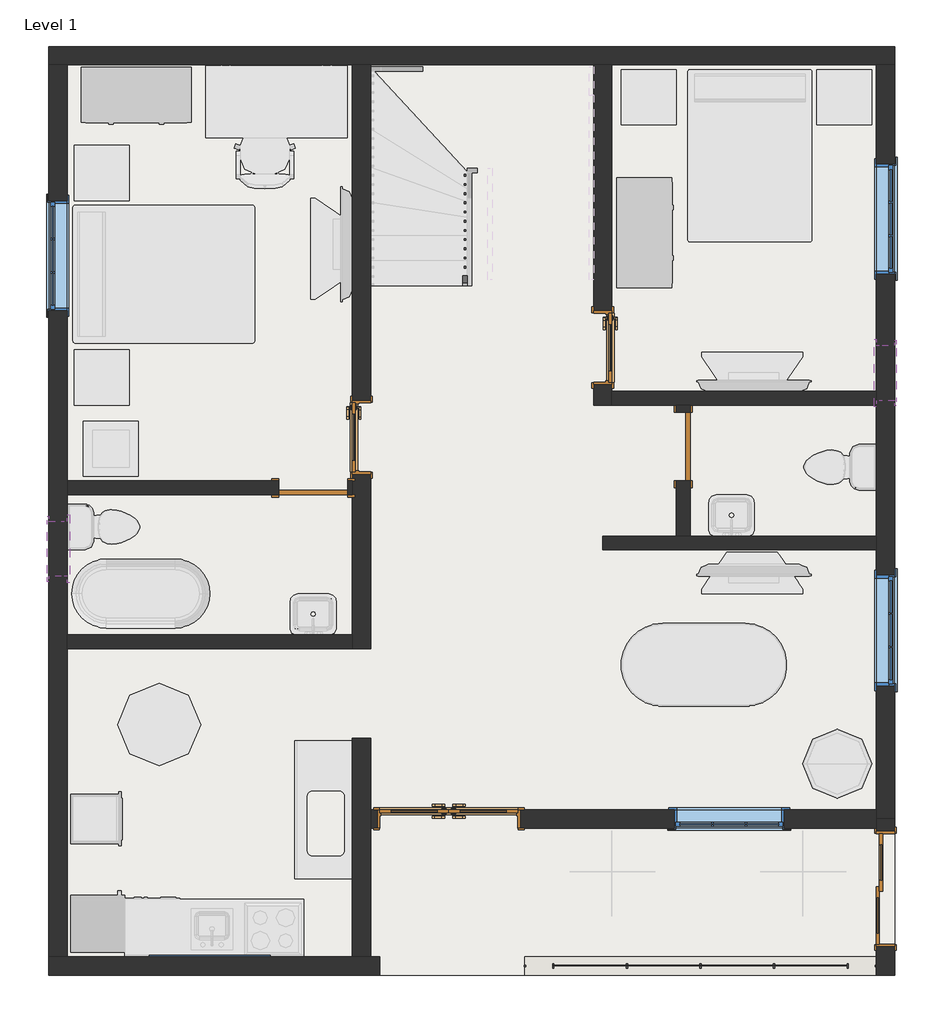
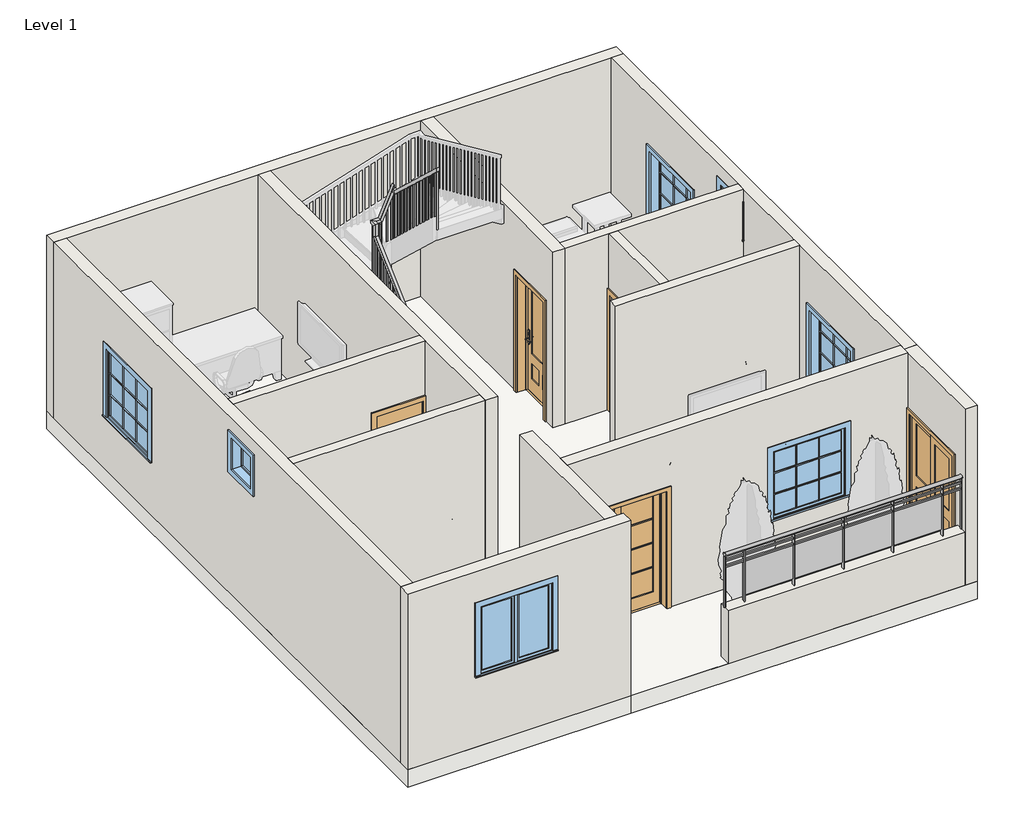
# One storey, part 1 of 2: 15 walls, 7 windows, 6 doors, 2 railings, 1 slab.
"""IFC4 building model written with IfcOpenShell, lengths in millimetres."""

from ifc_helpers import new_model, si_unit, point, frame, origin, origin_with_axes, place, context, project, spatial, polyline, ellipse_curve, trimmed, outline, extrude, faceted_brep, transform, mapped, element, save
from ifc_brep_helpers import plane_surface, extruded_surface, advanced_brep
from components import door_ad59dcae, door_41326d50, door_b03bd389, door_f9cb40a9, door_255cab33, window_3ea3e93d, window_0862ab64, window_e41d21a6

model = new_model("IFC4")

# Units and contexts
model_context = context("Model", 3, world=origin())
ifc_project = project(units=[si_unit("LENGTHUNIT", "METRE", prefix="MILLI")], contexts=[model_context])

# Site, building, storey
site = spatial("IfcSite", under=ifc_project)
building = spatial("IfcBuilding", under=site)
storey = spatial("IfcBuildingStorey", under=building, Name="Level 1", Elevation=0.0)

# Doors
placement = place(None, origin())
door_shape = door_ad59dcae(model_context)
element("IfcDoor", 1, ObjectType="30\" x 80\"", at=placement, inside=storey, context=model_context, shape_type="MappedRepresentation", body=[
    mapped(door_shape, transform((-8446.8361447, 7117.685558, 0.0), x_axis=(0.0, 1.0, 0.0), y_axis=(-1.0, 0.0, 0.0), z_axis=(0.0, 0.0, 1.0))),
])
door_2_shape = door_41326d50(model_context)
element("IfcDoor", 2, ObjectType="30\" x 80\"", at=placement, inside=storey, context=model_context, shape_type="MappedRepresentation", body=[
    mapped(door_2_shape, transform((-5773.4861447, 8108.285558, 0.0), x_axis=(0.0, 1.0, 0.0), y_axis=(-1.0, 0.0, 0.0), z_axis=(0.0, 0.0, 1.0))),
])
door_3_shape = door_b03bd389(model_context)
element("IfcDoor", 3, ObjectType="Door-Exterior-Double-Full Glass-Wood_Clad : 60\" x 80\"", at=placement, inside=storey, context=model_context, shape_type="MappedRepresentation", body=[
    mapped(door_3_shape, transform((-7478.4611447, 2904.460558, 0.0), x_axis=(1.0, 0.0, 0.0), y_axis=(0.0, 1.0, 0.0), z_axis=(0.0, 0.0, 1.0))),
])
door_4_shape = door_f9cb40a9(model_context)
element("IfcDoor", 4, ObjectType="Door-Interior-Double-Sliding-2_Panel-Wood : 48\" x 80\"", at=placement, inside=storey, context=model_context, shape_type="MappedRepresentation", body=[
    mapped(door_4_shape, transform((-2655.6361447, 2126.585558, 0.0), x_axis=(0.0, 1.0, 0.0), y_axis=(-1.0, 0.0, 0.0), z_axis=(0.0, 0.0, 1.0))),
])
door_5_shape = door_255cab33(model_context)
element("IfcDoor", 5, ObjectType="Single-Flush : 30\" x 80\"", at=placement, inside=storey, context=model_context, shape_type="MappedRepresentation", body=[
    mapped(door_5_shape, transform((-8977.0611447, 6558.885558, 0.0), x_axis=(1.0, 0.0, 0.0), y_axis=(0.0, 1.0, 0.0), z_axis=(0.0, 0.0, 1.0))),
])
element("IfcDoor", 6, ObjectType="Single-Flush : 30\" x 80\"", at=placement, inside=storey, context=model_context, shape_type="MappedRepresentation", body=[
    mapped(door_5_shape, transform((-4887.6611447, 7016.085558, 0.0), x_axis=(0.0, 1.0, 0.0), y_axis=(-1.0, 0.0, 0.0), z_axis=(0.0, 0.0, 1.0))),
])

# Railings
element("IfcRailing", 7, ObjectType="Glass Panel - Bottom Fill", at=placement, inside=storey, context=model_context, shape_type="SolidModel", body=[
    advanced_brep(
    [(-6640.2611447, 1313.785558, 1828.8), (-6640.2611447, 1237.585558, 1828.8), (-2754.0611447, 1313.785558, 1828.8), (-2754.0611447, 1237.585558, 1828.8)],
    [
        (0, 1, ellipse_curve(frame((-6640.2611447, 1275.685558, 1828.8), z_axis=(-1.0, 0.0, 0.0), x_axis=(0.0, -1.0, 0.0)), 38.1, 28.575)),
        (1, 0, ellipse_curve(frame((-6640.2611447, 1275.685558, 1828.8), z_axis=(-1.0, 0.0, 0.0), x_axis=(0.0, -1.0, 0.0)), 38.1, 28.575)),
        (2, 3, ellipse_curve(frame((-2754.0611447, 1275.685558, 1828.8), z_axis=(1.0, 0.0, 0.0), x_axis=(0.0, -1.0, 0.0)), 38.1, 28.575)),
        (3, 2, ellipse_curve(frame((-2754.0611447, 1275.685558, 1828.8), z_axis=(1.0, 0.0, 0.0), x_axis=(0.0, -1.0, 0.0)), 38.1, 28.575)),
        (0, 2),
        (3, 1),
    ],
    [
        plane_surface(frame((-6640.2611447, 1275.685558, 1828.8), z_axis=(-1.0, 0.0, 0.0), x_axis=(0.0, 1.0, 0.0))),
        plane_surface(frame((-2754.0611447, 1275.685558, 1828.8), z_axis=(1.0, 0.0, 0.0), x_axis=(0.0, 1.0, 0.0))),
        extruded_surface(trimmed(ellipse_curve(frame((-2754.0611447, 1275.685558, 1828.8), z_axis=(-1.0, 0.0, 0.0), x_axis=(0.0, -1.0, 0.0)), 38.1, 28.575), [point((-2754.0611447, 1313.785558, 1828.8))], [point((-2754.0611447, 1237.585558, 1828.8))], True, "CARTESIAN"), (-3886.2, 0.0, 0.0), 3886.2),
        extruded_surface(trimmed(ellipse_curve(frame((-2754.0611447, 1275.685558, 1828.8), z_axis=(-1.0, 0.0, 0.0), x_axis=(0.0, -1.0, 0.0)), 38.1, 28.575), [point((-2754.0611447, 1237.585558, 1828.8))], [point((-2754.0611447, 1313.785558, 1828.8))], True, "CARTESIAN"), (-3886.2, 0.0, 0.0), 3886.2),
    ],
    [
        (0, [[1, 2]]),
        (1, [[3, 4]]),
        (2, [[-1, 5, -4, 6]]),
        (3, [[-2, -6, -3, -5]]),
    ],
),
    extrude(outline(polyline([(-6640.2611447, 1262.985558), (-6640.2611447, 1288.385558), (-2754.0611447, 1288.385558), (-2754.0611447, 1262.985558), (-6640.2611447, 1262.985558)])), frame((0.0, 0.0, 1714.5), z_axis=(0.0, 0.0, 1.0), x_axis=(1.0, 0.0, 0.0)), (0.0, 0.0, 1.0), 25.4),
    extrude(outline(polyline([(-6640.2611447, 1262.985558), (-6640.2611447, 1288.385558), (-2754.0611447, 1288.385558), (-2754.0611447, 1262.985558), (-6640.2611447, 1262.985558)])), frame((0.0, 0.0, 1612.9), z_axis=(0.0, 0.0, 1.0), x_axis=(1.0, 0.0, 0.0)), (0.0, 0.0, 1.0), 25.4),
    extrude(outline(polyline([(-3077.9111447, 1250.285558), (-3077.9111447, 1301.085558), (-3065.2111447, 1301.085558), (-3065.2111447, 1250.285558), (-3077.9111447, 1250.285558)])), frame((0.0, 0.0, 914.4), z_axis=(0.0, 0.0, 1.0), x_axis=(1.0, 0.0, 0.0)), (0.0, 0.0, 1.0), 885.6788223),
    extrude(outline(polyline([(-3884.3611447, 1282.220715), (-3071.5611447, 1282.220715), (-3071.5611447, 1275.870715), (-3884.3611447, 1275.870715), (-3884.3611447, 1282.220715)])), frame((0.0, 0.0, 1016.0), z_axis=(0.0, 0.0, 1.0), x_axis=(1.0, 0.0, 0.0)), (0.0, 0.0, 1.0), 596.9),
    extrude(outline(polyline([(-3890.7111447, 1250.285558), (-3890.7111447, 1301.085558), (-3878.0111447, 1301.085558), (-3878.0111447, 1250.285558), (-3890.7111447, 1250.285558)])), frame((0.0, 0.0, 914.4), z_axis=(0.0, 0.0, 1.0), x_axis=(1.0, 0.0, 0.0)), (0.0, 0.0, 1.0), 885.6788223),
    extrude(outline(polyline([(-4697.1611447, 1282.220715), (-3884.3611447, 1282.220715), (-3884.3611447, 1275.870715), (-4697.1611447, 1275.870715), (-4697.1611447, 1282.220715)])), frame((0.0, 0.0, 1016.0), z_axis=(0.0, 0.0, 1.0), x_axis=(1.0, 0.0, 0.0)), (0.0, 0.0, 1.0), 596.9),
    extrude(outline(polyline([(-4703.5111447, 1250.285558), (-4703.5111447, 1301.085558), (-4690.8111447, 1301.085558), (-4690.8111447, 1250.285558), (-4703.5111447, 1250.285558)])), frame((0.0, 0.0, 914.4), z_axis=(0.0, 0.0, 1.0), x_axis=(1.0, 0.0, 0.0)), (0.0, 0.0, 1.0), 885.6788223),
    extrude(outline(polyline([(-5509.9611447, 1282.220715), (-4697.1611447, 1282.220715), (-4697.1611447, 1275.870715), (-5509.9611447, 1275.870715), (-5509.9611447, 1282.220715)])), frame((0.0, 0.0, 1016.0), z_axis=(0.0, 0.0, 1.0), x_axis=(1.0, 0.0, 0.0)), (0.0, 0.0, 1.0), 596.9),
    extrude(outline(polyline([(-5516.3111447, 1250.285558), (-5516.3111447, 1301.085558), (-5503.6111447, 1301.085558), (-5503.6111447, 1250.285558), (-5516.3111447, 1250.285558)])), frame((0.0, 0.0, 914.4), z_axis=(0.0, 0.0, 1.0), x_axis=(1.0, 0.0, 0.0)), (0.0, 0.0, 1.0), 885.6788223),
    extrude(outline(polyline([(-6322.7611447, 1282.220715), (-5509.9611447, 1282.220715), (-5509.9611447, 1275.870715), (-6322.7611447, 1275.870715), (-6322.7611447, 1282.220715)])), frame((0.0, 0.0, 1016.0), z_axis=(0.0, 0.0, 1.0), x_axis=(1.0, 0.0, 0.0)), (0.0, 0.0, 1.0), 596.9),
    extrude(outline(polyline([(-6329.1111447, 1250.285558), (-6329.1111447, 1301.085558), (-6316.4111447, 1301.085558), (-6316.4111447, 1250.285558), (-6329.1111447, 1250.285558)])), frame((0.0, 0.0, 914.4), z_axis=(0.0, 0.0, 1.0), x_axis=(1.0, 0.0, 0.0)), (0.0, 0.0, 1.0), 885.6788223),
    extrude(outline(polyline([(-2766.7611447, 1266.160558), (-2766.7611447, 1285.210558), (-2747.7111447, 1285.210558), (-2747.7111447, 1266.160558), (-2766.7611447, 1266.160558)])), frame((0.0, 0.0, 914.4), z_axis=(0.0, 0.0, 1.0), x_axis=(1.0, 0.0, 0.0)), (0.0, 0.0, 1.0), 885.6788223),
    extrude(outline(polyline([(-6646.6111447, 1266.160558), (-6646.6111447, 1285.210558), (-6627.5611447, 1285.210558), (-6627.5611447, 1266.160558), (-6646.6111447, 1266.160558)])), frame((0.0, 0.0, 914.4), z_axis=(0.0, 0.0, 1.0), x_axis=(1.0, 0.0, 0.0)), (0.0, 0.0, 1.0), 885.6788223),
])
element("IfcRailing", 8, ObjectType="Handrail - Rectangular", at=placement, inside=storey, context=model_context, shape_type="SolidModel", body=[
    faceted_brep([(-7326.0611447, 8794.085558, 1169.165648), (-7326.0611447, 8794.085558, 1100.6050042), (-7275.2611447, 8794.085558, 1100.6050042), (-7275.2611447, 8794.085558, 1169.165648), (-7326.0611447, 10017.0172498, 2277.570496), (-7326.0611447, 10067.8172498, 2255.0524616), (-7275.2611447, 10067.8172498, 2255.0524616), (-7275.2611447, 10017.0172498, 2277.570496), (-6970.4611447, 10144.0172498, 3008.8127173), (-6970.4611447, 10093.2172498, 3008.8127173), (-6970.4611447, 10093.2172498, 2882.2600622), (-6970.4611447, 10144.0172498, 2882.2600622), (-7165.8607082, 10144.0172498, 2436.4214755), (-7199.0611447, 10144.0172498, 2487.2214755), (-7165.8607082, 10093.2172498, 2436.4214755), (-7199.0611447, 10093.2172498, 2487.2214755), (-7326.0611447, 10017.0172498, 2487.2214755), (-7326.0611447, 10067.8172498, 2436.4214755), (-7275.2611447, 10067.8172498, 2436.4214755), (-7275.2611447, 10017.0172498, 2487.2214755), (-7326.0611447, 10144.0172498, 2487.2214755), (-7326.0611447, 10144.0172498, 2436.4214755), (-7275.2611447, 10093.2172498, 2436.4214755), (-7275.2611447, 10093.2172498, 2487.2214755)], [[[0, 1, 2, 3]], [[1, 0, 4, 5]], [[2, 1, 5, 6]], [[3, 2, 6, 7]], [[0, 3, 7, 4]], [[8, 9, 10, 11]], [[12, 13, 8, 11]], [[14, 12, 11, 10]], [[15, 14, 10, 9]], [[13, 15, 9, 8]], [[5, 4, 16, 17]], [[6, 5, 17, 18]], [[7, 6, 18, 19]], [[4, 7, 19, 16]], [[17, 16, 20, 21]], [[18, 17, 21, 22]], [[19, 18, 22, 23]], [[16, 19, 23, 20]], [[21, 20, 13, 12]], [[22, 21, 12, 14]], [[23, 22, 14, 15]], [[20, 23, 15, 13]]]),
    faceted_brep([(-6945.0611447, 8859.8360051, 4053.3777252), (-6995.8611447, 8859.8360051, 4053.3777252), (-6995.8611447, 8859.8360051, 3983.9464566), (-6945.0611447, 8859.8360051, 3983.9464566), (-6945.0611447, 10029.8112493, 2893.9053173), (-6945.0611447, 10049.8087726, 2944.7053173), (-6995.8611447, 10029.8112493, 2893.9053173), (-6995.8611447, 10049.8087726, 2944.7053173), (-6945.0611447, 10118.6172498, 2944.7053173), (-6945.0611447, 10118.6172498, 2893.9053173), (-6995.8611447, 10118.6172498, 2893.9053173), (-6995.8611447, 10118.6172498, 2944.7053173)], [[[0, 1, 2, 3]], [[4, 5, 0, 3]], [[6, 4, 3, 2]], [[7, 6, 2, 1]], [[5, 7, 1, 0]], [[8, 9, 10, 11]], [[9, 8, 5, 4]], [[10, 9, 4, 6]], [[11, 10, 6, 7]], [[8, 11, 7, 5]]]),
    extrude(outline(polyline([(8922.6837726, 3925.3925236), (8941.7337726, 3907.6440423), (8941.7337726, 2878.6666667), (8922.6837726, 2878.6666667), (8922.6837726, 3925.3925236)])), frame((-6979.9861447, 0.0, 0.0), z_axis=(1.0, 0.0, 0.0), x_axis=(0.0, 1.0, 0.0)), (0.0, 0.0, 1.0), 19.05),
    extrude(outline(polyline([(9024.2837726, 3830.7339569), (9043.3337726, 3812.9854756), (9043.3337726, 2878.6666667), (9024.2837726, 2878.6666667), (9024.2837726, 3830.7339569)])), frame((-6979.9861447, 0.0, 0.0), z_axis=(1.0, 0.0, 0.0), x_axis=(0.0, 1.0, 0.0)), (0.0, 0.0, 1.0), 19.05),
    extrude(outline(polyline([(9125.8837726, 3736.0753901), (9144.9337726, 3718.3269088), (9144.9337726, 2878.6666667), (9125.8837726, 2878.6666667), (9125.8837726, 3736.0753901)])), frame((-6979.9861447, 0.0, 0.0), z_axis=(1.0, 0.0, 0.0), x_axis=(0.0, 1.0, 0.0)), (0.0, 0.0, 1.0), 19.05),
    extrude(outline(polyline([(9227.4837726, 3641.4168233), (9246.5337726, 3623.6683421), (9246.5337726, 2709.3333333), (9227.4837726, 2709.3333333), (9227.4837726, 3641.4168233)])), frame((-6979.9861447, 0.0, 0.0), z_axis=(1.0, 0.0, 0.0), x_axis=(0.0, 1.0, 0.0)), (0.0, 0.0, 1.0), 19.05),
    extrude(outline(polyline([(9329.0837726, 3546.7582566), (9348.1337726, 3529.0097753), (9348.1337726, 2709.3333333), (9329.0837726, 2709.3333333), (9329.0837726, 3546.7582566)])), frame((-6979.9861447, 0.0, 0.0), z_axis=(1.0, 0.0, 0.0), x_axis=(0.0, 1.0, 0.0)), (0.0, 0.0, 1.0), 19.05),
    extrude(outline(polyline([(9430.6837726, 3452.0996898), (9449.7337726, 3434.3512086), (9449.7337726, 2540.0), (9430.6837726, 2540.0), (9430.6837726, 3452.0996898)])), frame((-6979.9861447, 0.0, 0.0), z_axis=(1.0, 0.0, 0.0), x_axis=(0.0, 1.0, 0.0)), (0.0, 0.0, 1.0), 19.05),
    extrude(outline(polyline([(9532.2837726, 3357.4411231), (9551.3337726, 3339.6926418), (9551.3337726, 2540.0), (9532.2837726, 2540.0), (9532.2837726, 3357.4411231)])), frame((-6979.9861447, 0.0, 0.0), z_axis=(1.0, 0.0, 0.0), x_axis=(0.0, 1.0, 0.0)), (0.0, 0.0, 1.0), 19.05),
    extrude(outline(polyline([(9633.8837726, 3262.7825563), (9652.9337726, 3245.0340751), (9652.9337726, 2370.6666667), (9633.8837726, 2370.6666667), (9633.8837726, 3262.7825563)])), frame((-6979.9861447, 0.0, 0.0), z_axis=(1.0, 0.0, 0.0), x_axis=(0.0, 1.0, 0.0)), (0.0, 0.0, 1.0), 19.05),
    extrude(outline(polyline([(9735.4837726, 3168.1239896), (9754.5337726, 3150.3755083), (9754.5337726, 2370.6666667), (9735.4837726, 2370.6666667), (9735.4837726, 3168.1239896)])), frame((-6979.9861447, 0.0, 0.0), z_axis=(1.0, 0.0, 0.0), x_axis=(0.0, 1.0, 0.0)), (0.0, 0.0, 1.0), 19.05),
    extrude(outline(polyline([(9837.0837726, 3073.4654228), (9856.1337726, 3055.7169415), (9856.1337726, 2201.3333333), (9837.0837726, 2201.3333333), (9837.0837726, 3073.4654228)])), frame((-6979.9861447, 0.0, 0.0), z_axis=(1.0, 0.0, 0.0), x_axis=(0.0, 1.0, 0.0)), (0.0, 0.0, 1.0), 19.05),
    extrude(outline(polyline([(9938.6837726, 2978.8068561), (9957.7337726, 2961.0583748), (9957.7337726, 2032.0), (9938.6837726, 2032.0), (9938.6837726, 2978.8068561)])), frame((-6979.9861447, 0.0, 0.0), z_axis=(1.0, 0.0, 0.0), x_axis=(0.0, 1.0, 0.0)), (0.0, 0.0, 1.0), 19.05),
    extrude(outline(polyline([(2671.3464031, -7062.8991663), (2627.8804663, -7081.9491663), (1693.3333333, -7081.9491663), (1693.3333333, -7062.8991663), (2671.3464031, -7062.8991663)])), frame((0.0, 10109.0922498, 0.0), z_axis=(0.0, 1.0, 0.0), x_axis=(0.0, 0.0, 1.0)), (0.0, 0.0, 1.0), 19.05),
    extrude(outline(polyline([(2439.5280734, -7164.4991663), (2396.0621366, -7183.5491663), (1524.0, -7183.5491663), (1524.0, -7164.4991663), (2439.5280734, -7164.4991663)])), frame((0.0, 10109.0922498, 0.0), z_axis=(0.0, 1.0, 0.0), x_axis=(0.0, 0.0, 1.0)), (0.0, 0.0, 1.0), 19.05),
    extrude(outline(polyline([(10003.760558, 2196.9946418), (10022.810558, 2214.2606203), (10022.810558, 1185.3333333), (10003.760558, 1185.3333333), (10003.760558, 2196.9946418)])), frame((-7310.1861447, 0.0, 0.0), z_axis=(1.0, 0.0, 0.0), x_axis=(0.0, 1.0, 0.0)), (0.0, 0.0, 1.0), 19.05),
    extrude(outline(polyline([(9902.160558, 2104.9094229), (9921.210558, 2122.1754014), (9921.210558, 1185.3333333), (9902.160558, 1185.3333333), (9902.160558, 2104.9094229)])), frame((-7310.1861447, 0.0, 0.0), z_axis=(1.0, 0.0, 0.0), x_axis=(0.0, 1.0, 0.0)), (0.0, 0.0, 1.0), 19.05),
    extrude(outline(polyline([(9800.560558, 2012.824204), (9819.610558, 2030.0901825), (9819.610558, 1016.0), (9800.560558, 1016.0), (9800.560558, 2012.824204)])), frame((-7310.1861447, 0.0, 0.0), z_axis=(1.0, 0.0, 0.0), x_axis=(0.0, 1.0, 0.0)), (0.0, 0.0, 1.0), 19.05),
    extrude(outline(polyline([(9698.960558, 1920.738985), (9718.010558, 1938.0049636), (9718.010558, 846.6666667), (9698.960558, 846.6666667), (9698.960558, 1920.738985)])), frame((-7310.1861447, 0.0, 0.0), z_axis=(1.0, 0.0, 0.0), x_axis=(0.0, 1.0, 0.0)), (0.0, 0.0, 1.0), 19.05),
    extrude(outline(polyline([(9597.360558, 1828.6537661), (9616.410558, 1845.9197447), (9616.410558, 846.6666667), (9597.360558, 846.6666667), (9597.360558, 1828.6537661)])), frame((-7310.1861447, 0.0, 0.0), z_axis=(1.0, 0.0, 0.0), x_axis=(0.0, 1.0, 0.0)), (0.0, 0.0, 1.0), 19.05),
    extrude(outline(polyline([(9495.760558, 1736.5685472), (9514.810558, 1753.8345258), (9514.810558, 677.3333333), (9495.760558, 677.3333333), (9495.760558, 1736.5685472)])), frame((-7310.1861447, 0.0, 0.0), z_axis=(1.0, 0.0, 0.0), x_axis=(0.0, 1.0, 0.0)), (0.0, 0.0, 1.0), 19.05),
    extrude(outline(polyline([(9394.160558, 1644.4833283), (9413.210558, 1661.7493069), (9413.210558, 677.3333333), (9394.160558, 677.3333333), (9394.160558, 1644.4833283)])), frame((-7310.1861447, 0.0, 0.0), z_axis=(1.0, 0.0, 0.0), x_axis=(0.0, 1.0, 0.0)), (0.0, 0.0, 1.0), 19.05),
    extrude(outline(polyline([(9292.560558, 1552.3981094), (9311.610558, 1569.664088), (9311.610558, 508.0), (9292.560558, 508.0), (9292.560558, 1552.3981094)])), frame((-7310.1861447, 0.0, 0.0), z_axis=(1.0, 0.0, 0.0), x_axis=(0.0, 1.0, 0.0)), (0.0, 0.0, 1.0), 19.05),
    extrude(outline(polyline([(9190.960558, 1460.3128905), (9210.010558, 1477.5788691), (9210.010558, 508.0), (9190.960558, 508.0), (9190.960558, 1460.3128905)])), frame((-7310.1861447, 0.0, 0.0), z_axis=(1.0, 0.0, 0.0), x_axis=(0.0, 1.0, 0.0)), (0.0, 0.0, 1.0), 19.05),
    extrude(outline(polyline([(9089.360558, 1368.2276716), (9108.410558, 1385.4936501), (9108.410558, 508.0), (9089.360558, 508.0), (9089.360558, 1368.2276716)])), frame((-7310.1861447, 0.0, 0.0), z_axis=(1.0, 0.0, 0.0), x_axis=(0.0, 1.0, 0.0)), (0.0, 0.0, 1.0), 19.05),
    extrude(outline(polyline([(8987.760558, 1276.1424527), (9006.810558, 1293.4084312), (9006.810558, 338.6666667), (8987.760558, 338.6666667), (8987.760558, 1276.1424527)])), frame((-7310.1861447, 0.0, 0.0), z_axis=(1.0, 0.0, 0.0), x_axis=(0.0, 1.0, 0.0)), (0.0, 0.0, 1.0), 19.05),
    extrude(outline(polyline([(8886.160558, 1184.0572338), (8905.210558, 1201.3232123), (8905.210558, 338.6666667), (8886.160558, 338.6666667), (8886.160558, 1184.0572338)])), frame((-7310.1861447, 0.0, 0.0), z_axis=(1.0, 0.0, 0.0), x_axis=(0.0, 1.0, 0.0)), (0.0, 0.0, 1.0), 19.05),
    extrude(outline(polyline([(-6979.9861447, 10059.3337726), (-6960.9361447, 10059.3337726), (-6960.9361447, 10040.2837726), (-6979.9861447, 10040.2837726), (-6979.9861447, 10059.3337726)])), frame((0.0, 0.0, 2032.0), z_axis=(0.0, 0.0, 1.0), x_axis=(1.0, 0.0, 0.0)), (0.0, 0.0, 1.0), 861.9053173),
    extrude(outline(polyline([(2903.9930306, -6960.9361447), (2860.5270938, -6979.9861447), (1862.6666667, -6979.9861447), (1862.6666667, -6960.9361447), (2903.9930306, -6960.9361447)])), frame((0.0, 10109.0922498, 0.0), z_axis=(0.0, 1.0, 0.0), x_axis=(0.0, 0.0, 1.0)), (0.0, 0.0, 1.0), 19.05),
    extrude(outline(polyline([(2839.8856307, -6989.0327661), (2796.4196939, -7008.0827661), (1862.6666667, -7008.0827661), (1862.6666667, -6989.0327661), (2839.8856307, -6989.0327661)])), frame((0.0, 10109.0922498, 0.0), z_axis=(0.0, 1.0, 0.0), x_axis=(0.0, 0.0, 1.0)), (0.0, 0.0, 1.0), 19.05),
    extrude(outline(polyline([(-7285.1491663, 10109.0922498), (-7285.1491663, 10128.1422498), (-7266.0991663, 10128.1422498), (-7266.0991663, 10109.0922498), (-7285.1491663, 10109.0922498)])), frame((0.0, 0.0, 1354.6666667), z_axis=(0.0, 0.0, 1.0), x_axis=(1.0, 0.0, 0.0)), (0.0, 0.0, 1.0), 1081.7548088),
    extrude(outline(polyline([(-7291.1361447, 10109.0922498), (-7310.1861447, 10109.0922498), (-7310.1861447, 10128.1422498), (-7291.1361447, 10128.1422498), (-7291.1361447, 10109.0922498)])), frame((0.0, 0.0, 1354.6666667), z_axis=(0.0, 0.0, 1.0), x_axis=(1.0, 0.0, 0.0)), (0.0, 0.0, 1.0), 1081.7548088),
    extrude(outline(polyline([(-7291.1361447, 10046.0633449), (-7310.1861447, 10046.0633449), (-7310.1861447, 10065.1133449), (-7291.1361447, 10065.1133449), (-7291.1361447, 10046.0633449)])), frame((0.0, 0.0, 1354.6666667), z_axis=(0.0, 0.0, 1.0), x_axis=(1.0, 0.0, 0.0)), (0.0, 0.0, 1.0), 872.1038293),
    extrude(outline(polyline([(8859.8360051, 3983.9464566), (8878.8860051, 3966.1979753), (8878.8860051, 2878.6666667), (8859.8360051, 2878.6666667), (8859.8360051, 3983.9464566)])), frame((-6979.9861447, 0.0, 0.0), z_axis=(1.0, 0.0, 0.0), x_axis=(0.0, 1.0, 0.0)), (0.0, 0.0, 1.0), 19.05),
    extrude(outline(polyline([(8794.085558, 1100.6050042), (8813.135558, 1117.8709827), (8813.135558, 338.6666667), (8794.085558, 338.6666667), (8794.085558, 1100.6050042)])), frame((-7310.1861447, 0.0, 0.0), z_axis=(1.0, 0.0, 0.0), x_axis=(0.0, 1.0, 0.0)), (0.0, 0.0, 1.0), 19.05),
])

# Slab
element("IfcSlab", 9, ObjectType="Generic - 12\"", at=placement, inside=storey, context=model_context, shape_type="SweptSolid", body=[
    extrude(outline(polyline([(-2550.8611447, 11435.685558), (-2550.8611447, 2806.035558), (-2550.8611447, 1174.085558), (-8240.4611447, 1174.085558), (-11898.0611447, 1174.085558), (-11898.0611447, 11435.685558), (-2550.8611447, 11435.685558)])), frame((0.0, 0.0, -304.8), z_axis=(0.0, 0.0, 1.0), x_axis=(1.0, 0.0, 0.0)), (0.0, 0.0, 1.0), 304.8),
])

# Walls
element("IfcWall", 10, ObjectType="Generic - 8\"", at=placement, inside=storey, context=model_context, shape_type="Brep", body=[
    faceted_brep([(-11898.0611447, 11232.485558, 0.0), (-11694.8611447, 11232.485558, 0.0), (-8545.2611447, 11232.485558, 0.0), (-8342.0611447, 11232.485558, 0.0), (-5878.2611447, 11232.485558, 0.0), (-5675.0611447, 11232.485558, 0.0), (-2754.0611447, 11232.485558, 0.0), (-2550.8611447, 11232.485558, 0.0), (-2550.8611447, 11232.485558, 3048.0), (-2754.0611447, 11232.485558, 3048.0), (-5675.0611447, 11232.485558, 3048.0), (-5878.2611447, 11232.485558, 3048.0), (-8342.0611447, 11232.485558, 3048.0), (-8545.2611447, 11232.485558, 3048.0), (-11694.8611447, 11232.485558, 3048.0), (-11898.0611447, 11232.485558, 3048.0), (-11898.0611447, 11435.685558, 0.0), (-11898.0611447, 11435.685558, 3048.0), (-2550.8611447, 11435.685558, 3048.0), (-2550.8611447, 11435.685558, 0.0)], [[[0, 1, 2, 3, 4, 5, 6, 7, 8, 9, 10, 11, 12, 13, 14, 15]], [[16, 17, 18, 19]], [[7, 6, 5, 4, 3, 2, 1, 0, 16, 19]], [[8, 7, 19, 18]], [[0, 15, 17, 16]], [[15, 14, 13, 12, 11, 10, 9, 8, 18, 17]]]),
])
element("IfcWall", 11, ObjectType="Generic - 8\"", at=placement, inside=storey, context=model_context, shape_type="Brep", body=[
    faceted_brep([(-2754.0611447, 11232.485558, 0.0), (-2754.0611447, 7625.685558, 0.0), (-2754.0611447, 7473.285558, 0.0), (-2754.0611447, 6025.485558, 0.0), (-2754.0611447, 5873.085558, 0.0), (-2754.0611447, 3002.885558, 0.0), (-2754.0611447, 2901.285558, 0.0), (-2754.0611447, 2901.285558, 3048.0), (-2754.0611447, 3002.885558, 3048.0), (-2754.0611447, 5873.085558, 3048.0), (-2754.0611447, 6025.485558, 3048.0), (-2754.0611447, 7473.285558, 3048.0), (-2754.0611447, 7625.685558, 3048.0), (-2754.0611447, 11232.485558, 3048.0), (-2754.0611447, 4374.485558, 2133.6), (-2754.0611447, 4374.485558, 914.4), (-2754.0611447, 5593.685558, 914.4), (-2754.0611447, 5593.685558, 2133.6), (-2754.0611447, 8921.085558, 2133.6), (-2754.0611447, 8921.085558, 914.4), (-2754.0611447, 10140.285558, 914.4), (-2754.0611447, 10140.285558, 2133.6), (-2754.0611447, 8133.685558, 2768.6), (-2754.0611447, 7524.085558, 2768.6), (-2754.0611447, 7524.085558, 2159.0), (-2754.0611447, 8133.685558, 2159.0), (-2550.8611447, 11232.485558, 0.0), (-2550.8611447, 11232.485558, 3048.0), (-2550.8611447, 2901.285558, 3048.0), (-2550.8611447, 2901.285558, 0.0), (-2550.8611447, 4374.485558, 2133.6), (-2550.8611447, 5593.685558, 2133.6), (-2550.8611447, 5593.685558, 914.4), (-2550.8611447, 4374.485558, 914.4), (-2550.8611447, 8921.085558, 2133.6), (-2550.8611447, 10140.285558, 2133.6), (-2550.8611447, 10140.285558, 914.4), (-2550.8611447, 8921.085558, 914.4), (-2550.8611447, 8133.685558, 2768.6), (-2550.8611447, 8133.685558, 2159.0), (-2550.8611447, 7524.085558, 2159.0), (-2550.8611447, 7524.085558, 2768.6)], [[[0, 1, 2, 3, 4, 5, 6, 7, 8, 9, 10, 11, 12, 13], [14, 15, 16, 17], [18, 19, 20, 21], [22, 23, 24, 25]], [[26, 27, 28, 29], [30, 31, 32, 33], [34, 35, 36, 37], [38, 39, 40, 41]], [[6, 5, 4, 3, 2, 1, 0, 26, 29]], [[7, 6, 29, 28]], [[0, 13, 27, 26]], [[15, 14, 30, 33]], [[16, 15, 33, 32]], [[17, 16, 32, 31]], [[14, 17, 31, 30]], [[19, 18, 34, 37]], [[20, 19, 37, 36]], [[21, 20, 36, 35]], [[18, 21, 35, 34]], [[39, 38, 22, 25]], [[40, 39, 25, 24]], [[41, 40, 24, 23]], [[38, 41, 23, 22]], [[13, 12, 11, 10, 9, 8, 7, 28, 27]]]),
])
element("IfcWall", 12, ObjectType="Generic - 8\"", at=placement, inside=storey, context=model_context, shape_type="SweptSolid", body=[
    extrude(outline(polyline([(-6640.2611447, 1377.285558), (-2754.0611447, 1377.285558), (-2754.0611447, 1174.085558), (-6640.2611447, 1174.085558), (-6640.2611447, 1377.285558)])), origin_with_axes(), (0.0, 0.0, 1.0), 914.4),
])
element("IfcWall", 13, ObjectType="Generic - 8\"", at=placement, inside=storey, context=model_context, shape_type="Brep", body=[
    faceted_brep([(-11694.8611447, 1377.285558, 0.0), (-11694.8611447, 4780.885558, 0.0), (-11694.8611447, 4933.285558, 0.0), (-11694.8611447, 6482.685558, 0.0), (-11694.8611447, 6635.085558, 0.0), (-11694.8611447, 11232.485558, 0.0), (-11694.8611447, 11232.485558, 3048.0), (-11694.8611447, 6635.085558, 3048.0), (-11694.8611447, 6482.685558, 3048.0), (-11694.8611447, 4933.285558, 3048.0), (-11694.8611447, 4780.885558, 3048.0), (-11694.8611447, 1377.285558, 3048.0), (-11694.8611447, 9733.885558, 2133.6), (-11694.8611447, 9733.885558, 914.4), (-11694.8611447, 8514.685558, 914.4), (-11694.8611447, 8514.685558, 2133.6), (-11694.8611447, 5580.985558, 2768.6), (-11694.8611447, 6190.585558, 2768.6), (-11694.8611447, 6190.585558, 2159.0), (-11694.8611447, 5580.985558, 2159.0), (-11898.0611447, 1377.285558, 0.0), (-11898.0611447, 1377.285558, 3048.0), (-11898.0611447, 11232.485558, 3048.0), (-11898.0611447, 11232.485558, 0.0), (-11898.0611447, 9733.885558, 2133.6), (-11898.0611447, 8514.685558, 2133.6), (-11898.0611447, 8514.685558, 914.4), (-11898.0611447, 9733.885558, 914.4), (-11898.0611447, 5580.985558, 2768.6), (-11898.0611447, 5580.985558, 2159.0), (-11898.0611447, 6190.585558, 2159.0), (-11898.0611447, 6190.585558, 2768.6)], [[[0, 1, 2, 3, 4, 5, 6, 7, 8, 9, 10, 11], [12, 13, 14, 15], [16, 17, 18, 19]], [[20, 21, 22, 23], [24, 25, 26, 27], [28, 29, 30, 31]], [[5, 4, 3, 2, 1, 0, 20, 23]], [[6, 5, 23, 22]], [[0, 11, 21, 20]], [[13, 12, 24, 27]], [[14, 13, 27, 26]], [[15, 14, 26, 25]], [[12, 15, 25, 24]], [[29, 28, 16, 19]], [[30, 29, 19, 18]], [[31, 30, 18, 17]], [[28, 31, 17, 16]], [[11, 10, 9, 8, 7, 6, 22, 21]]]),
])
element("IfcWall", 14, ObjectType="Generic - 8\"", at=placement, inside=storey, context=model_context, shape_type="Brep", body=[
    faceted_brep([(-8342.0611447, 1377.285558, 0.0), (-8342.0611447, 2799.685558, 0.0), (-8342.0611447, 3002.885558, 0.0), (-8342.0611447, 3790.285558, 0.0), (-8342.0611447, 3790.285558, 3048.0), (-8342.0611447, 3002.885558, 3048.0), (-8342.0611447, 2799.685558, 3048.0), (-8342.0611447, 1377.285558, 3048.0), (-8545.2611447, 1377.285558, 0.0), (-8545.2611447, 1377.285558, 3048.0), (-8545.2611447, 3790.285558, 3048.0), (-8545.2611447, 3790.285558, 0.0)], [[[0, 1, 2, 3, 4, 5, 6, 7]], [[8, 9, 10, 11]], [[3, 2, 1, 0, 8, 11]], [[4, 3, 11, 10]], [[0, 7, 9, 8]], [[7, 6, 5, 4, 10, 9]]]),
])
element("IfcWall", 15, ObjectType="Generic - 8\"", at=placement, inside=storey, context=model_context, shape_type="Brep", body=[
    faceted_brep([(-8342.0611447, 2799.685558, 3048.0), (-8342.0611447, 2799.685558, 0.0), (-8265.8611447, 2799.685558, 0.0), (-8265.8611447, 2799.685558, 2057.4), (-6691.0611447, 2799.685558, 2057.4), (-6691.0611447, 2799.685558, 0.0), (-2754.0611447, 2799.685558, 0.0), (-2754.0611447, 2799.685558, 3048.0), (-4989.2611447, 2799.685558, 2133.6), (-3770.0611447, 2799.685558, 2133.6), (-3770.0611447, 2799.685558, 914.4), (-4989.2611447, 2799.685558, 914.4), (-8342.0611447, 3002.885558, 0.0), (-8342.0611447, 3002.885558, 3048.0), (-2754.0611447, 3002.885558, 3048.0), (-2754.0611447, 3002.885558, 0.0), (-6691.0611447, 3002.885558, 0.0), (-6691.0611447, 3002.885558, 2057.4), (-8265.8611447, 3002.885558, 2057.4), (-8265.8611447, 3002.885558, 0.0), (-4989.2611447, 3002.885558, 2133.6), (-4989.2611447, 3002.885558, 914.4), (-3770.0611447, 3002.885558, 914.4), (-3770.0611447, 3002.885558, 2133.6), (-2754.0611447, 2901.285558, 0.0), (-2754.0611447, 2901.285558, 3048.0)], [[[0, 1, 2, 3, 4, 5, 6, 7], [8, 9, 10, 11]], [[12, 13, 14, 15, 16, 17, 18, 19], [20, 21, 22, 23]], [[1, 12, 19, 2]], [[15, 24, 6, 5, 16]], [[1, 0, 13, 12]], [[4, 17, 16, 5]], [[17, 4, 3, 18]], [[18, 3, 2, 19]], [[7, 6, 24, 15, 14, 25]], [[21, 20, 8, 11]], [[22, 21, 11, 10]], [[23, 22, 10, 9]], [[20, 23, 9, 8]], [[0, 7, 25, 14, 13]]]),
])
element("IfcWall", 16, ObjectType="Generic - 8\"", at=placement, inside=storey, context=model_context, shape_type="Brep", body=[
    faceted_brep([(-5878.2611447, 11232.485558, 3048.0), (-5878.2611447, 11232.485558, 0.0), (-5878.2611447, 8514.685558, 0.0), (-5878.2611447, 8514.685558, 2057.4), (-5878.2611447, 7701.885558, 2057.4), (-5878.2611447, 7701.885558, 0.0), (-5878.2611447, 7473.285558, 0.0), (-5878.2611447, 7473.285558, 3048.0), (-5675.0611447, 11232.485558, 0.0), (-5675.0611447, 11232.485558, 3048.0), (-5675.0611447, 7625.685558, 3048.0), (-5675.0611447, 7473.285558, 3048.0), (-5675.0611447, 7473.285558, 0.0), (-5675.0611447, 7625.685558, 0.0), (-5675.0611447, 7701.885558, 0.0), (-5675.0611447, 7701.885558, 2057.4), (-5675.0611447, 8514.685558, 2057.4), (-5675.0611447, 8514.685558, 0.0)], [[[0, 1, 2, 3, 4, 5, 6, 7]], [[8, 9, 10, 11, 12, 13, 14, 15, 16, 17]], [[1, 8, 17, 2]], [[12, 6, 5, 14, 13]], [[1, 0, 9, 8]], [[7, 6, 12, 11]], [[16, 3, 2, 17]], [[3, 16, 15, 4]], [[4, 15, 14, 5]], [[0, 7, 11, 10, 9]]]),
])
element("IfcWall", 17, ObjectType="Generic - 8\"", at=placement, inside=storey, context=model_context, shape_type="Brep", body=[
    faceted_brep([(-8342.0611447, 11232.485558, 0.0), (-8342.0611447, 11232.485558, 3048.0), (-8342.0611447, 4780.885558, 3048.0), (-8342.0611447, 4780.885558, 0.0), (-8342.0611447, 6711.285558, 0.0), (-8342.0611447, 6711.285558, 2057.4), (-8342.0611447, 7524.085558, 2057.4), (-8342.0611447, 7524.085558, 0.0), (-8545.2611447, 11232.485558, 3048.0), (-8545.2611447, 11232.485558, 0.0), (-8545.2611447, 7524.085558, 0.0), (-8545.2611447, 7524.085558, 2057.4), (-8545.2611447, 6711.285558, 2057.4), (-8545.2611447, 6711.285558, 0.0), (-8545.2611447, 6635.085558, 0.0), (-8545.2611447, 6482.685558, 0.0), (-8545.2611447, 4933.285558, 0.0), (-8545.2611447, 4780.885558, 0.0), (-8545.2611447, 4780.885558, 3048.0), (-8545.2611447, 4933.285558, 3048.0), (-8545.2611447, 6482.685558, 3048.0), (-8545.2611447, 6635.085558, 3048.0)], [[[0, 1, 2, 3, 4, 5, 6, 7]], [[8, 9, 10, 11, 12, 13, 14, 15, 16, 17, 18, 19, 20, 21]], [[9, 0, 7, 10]], [[3, 17, 16, 15, 14, 13, 4]], [[1, 0, 9, 8]], [[3, 2, 18, 17]], [[6, 11, 10, 7]], [[11, 6, 5, 12]], [[12, 5, 4, 13]], [[2, 1, 8, 21, 20, 19, 18]]]),
])
element("IfcWall", 18, ObjectType="Generic - 8\"", at=placement, inside=storey, context=model_context, shape_type="Brep", body=[
    faceted_brep([(-8240.4611447, 1377.285558, 0.0), (-8342.0611447, 1377.285558, 0.0), (-8545.2611447, 1377.285558, 0.0), (-11694.8611447, 1377.285558, 0.0), (-11898.0611447, 1377.285558, 0.0), (-11898.0611447, 1377.285558, 3048.0), (-11694.8611447, 1377.285558, 3048.0), (-8545.2611447, 1377.285558, 3048.0), (-8342.0611447, 1377.285558, 3048.0), (-8240.4611447, 1377.285558, 3048.0), (-10729.6611447, 1377.285558, 2438.4), (-10729.6611447, 1377.285558, 1219.2), (-9510.4611447, 1377.285558, 1219.2), (-9510.4611447, 1377.285558, 2438.4), (-8240.4611447, 1174.085558, 0.0), (-8240.4611447, 1174.085558, 3048.0), (-11898.0611447, 1174.085558, 3048.0), (-11898.0611447, 1174.085558, 0.0), (-10729.6611447, 1174.085558, 2438.4), (-9510.4611447, 1174.085558, 2438.4), (-9510.4611447, 1174.085558, 1219.2), (-10729.6611447, 1174.085558, 1219.2)], [[[0, 1, 2, 3, 4, 5, 6, 7, 8, 9], [10, 11, 12, 13]], [[14, 15, 16, 17], [18, 19, 20, 21]], [[4, 3, 2, 1, 0, 14, 17]], [[0, 9, 15, 14]], [[5, 4, 17, 16]], [[11, 10, 18, 21]], [[12, 11, 21, 20]], [[13, 12, 20, 19]], [[10, 13, 19, 18]], [[9, 8, 7, 6, 5, 16, 15]]]),
])
element("IfcWall", 19, ObjectType="Generic - 8\"", at=placement, inside=storey, context=model_context, shape_type="Brep", body=[
    faceted_brep([(-2754.0611447, 2901.285558, 3048.0), (-2754.0611447, 2901.285558, 0.0), (-2754.0611447, 2799.685558, 0.0), (-2754.0611447, 2761.585558, 0.0), (-2754.0611447, 2761.585558, 2057.4), (-2754.0611447, 1491.585558, 2057.4), (-2754.0611447, 1491.585558, 0.0), (-2754.0611447, 1377.285558, 0.0), (-2754.0611447, 1174.085558, 0.0), (-2754.0611447, 1174.085558, 914.4), (-2754.0611447, 1174.085558, 3048.0), (-2754.0611447, 2799.685558, 3048.0), (-2550.8611447, 2901.285558, 0.0), (-2550.8611447, 2901.285558, 3048.0), (-2550.8611447, 1174.085558, 3048.0), (-2550.8611447, 1174.085558, 0.0), (-2550.8611447, 1491.585558, 0.0), (-2550.8611447, 1491.585558, 2057.4), (-2550.8611447, 2761.585558, 2057.4), (-2550.8611447, 2761.585558, 0.0)], [[[0, 1, 2, 3, 4, 5, 6, 7, 8, 9, 10, 11]], [[12, 13, 14, 15, 16, 17, 18, 19]], [[15, 8, 7, 6, 16]], [[1, 12, 19, 3, 2]], [[1, 0, 13, 12]], [[10, 9, 8, 15, 14]], [[18, 4, 3, 19]], [[4, 18, 17, 5]], [[5, 17, 16, 6]], [[0, 11, 10, 14, 13]]]),
])
element("IfcWall", 20, ObjectType="INNER WALL", at=placement, inside=storey, context=model_context, shape_type="SweptSolid", body=[
    extrude(outline(polyline([(-11694.8611447, 4933.285558), (-8545.2611447, 4933.285558), (-8545.2611447, 4780.885558), (-11694.8611447, 4780.885558), (-11694.8611447, 4933.285558)])), origin_with_axes(), (0.0, 0.0, 1.0), 3048.0),
])
element("IfcWall", 21, ObjectType="INNER WALL", at=placement, inside=storey, context=model_context, shape_type="SweptSolid", body=[
    extrude(outline(polyline([(2032.0, -8596.0611447), (0.0, -8596.0611447), (0.0, -8545.2611447), (3048.0, -8545.2611447), (3048.0, -11694.8611447), (0.0, -11694.8611447), (0.0, -9358.0611447), (2032.0, -9358.0611447), (2032.0, -8596.0611447)])), frame((0.0, 6482.685558, 0.0), z_axis=(0.0, 1.0, 0.0), x_axis=(0.0, 0.0, 1.0)), (0.0, 0.0, 1.0), 152.4),
])
element("IfcWall", 22, ObjectType="INNER WALL", at=placement, inside=storey, context=model_context, shape_type="Brep", body=[
    faceted_brep([(-5776.6611447, 5873.085558, 0.0), (-2754.0611447, 5873.085558, 0.0), (-2754.0611447, 5873.085558, 3048.0), (-5776.6611447, 5873.085558, 3048.0), (-5776.6611447, 6025.485558, 0.0), (-5776.6611447, 6025.485558, 3048.0), (-4963.8611447, 6025.485558, 3048.0), (-4811.4611447, 6025.485558, 3048.0), (-2754.0611447, 6025.485558, 3048.0), (-2754.0611447, 6025.485558, 0.0), (-4811.4611447, 6025.485558, 0.0), (-4963.8611447, 6025.485558, 0.0)], [[[0, 1, 2, 3]], [[4, 5, 6, 7, 8, 9, 10, 11]], [[1, 0, 4, 11, 10, 9]], [[0, 3, 5, 4]], [[2, 1, 9, 8]], [[3, 2, 8, 7, 6, 5]]]),
])
element("IfcWall", 23, ObjectType="INNER WALL", at=placement, inside=storey, context=model_context, shape_type="Brep", body=[
    faceted_brep([(-2754.0611447, 7625.685558, 0.0), (-5675.0611447, 7625.685558, 0.0), (-5675.0611447, 7625.685558, 3048.0), (-2754.0611447, 7625.685558, 3048.0), (-2754.0611447, 7473.285558, 0.0), (-2754.0611447, 7473.285558, 3048.0), (-4811.4611447, 7473.285558, 3048.0), (-4963.8611447, 7473.285558, 3048.0), (-5675.0611447, 7473.285558, 3048.0), (-5675.0611447, 7473.285558, 0.0), (-4963.8611447, 7473.285558, 0.0), (-4811.4611447, 7473.285558, 0.0)], [[[0, 1, 2, 3]], [[4, 5, 6, 7, 8, 9, 10, 11]], [[1, 0, 4, 11, 10, 9]], [[0, 3, 5, 4]], [[2, 1, 9, 8]], [[3, 2, 8, 7, 6, 5]]]),
])
element("IfcWall", 24, ObjectType="INNER WALL", at=placement, inside=storey, context=model_context, shape_type="SweptSolid", body=[
    extrude(outline(polyline([(6025.485558, 0.0), (6025.485558, 3048.0), (7473.285558, 3048.0), (7473.285558, 0.0), (7397.085558, 0.0), (7397.085558, 2032.0), (6635.085558, 2032.0), (6635.085558, 0.0), (6025.485558, 0.0)])), frame((-4963.8611447, 0.0, 0.0), z_axis=(1.0, 0.0, 0.0), x_axis=(0.0, 1.0, 0.0)), (0.0, 0.0, 1.0), 152.4),
])

# Windows
window_shape = window_3ea3e93d(model_context)
element("IfcWindow", 25, ObjectType="Casement 3x3 with Trim : 48\" x 48\"", at=placement, inside=storey, context=model_context, shape_type="MappedRepresentation", body=[
    mapped(window_shape, transform((-4379.6611447, 2901.285558, 304.8), x_axis=(-1.0, 0.0, 0.0), y_axis=(0.0, -1.0, 0.0), z_axis=(0.0, 0.0, 1.0))),
])
element("IfcWindow", 26, ObjectType="Casement 3x3 with Trim : 48\" x 48\"", at=placement, inside=storey, context=model_context, shape_type="MappedRepresentation", body=[
    mapped(window_shape, transform((-2652.4611447, 4984.085558, 304.8), x_axis=(0.0, -1.0, 0.0), y_axis=(1.0, 0.0, 0.0), z_axis=(0.0, 0.0, 1.0))),
])
element("IfcWindow", 27, ObjectType="Casement 3x3 with Trim : 48\" x 48\"", at=placement, inside=storey, context=model_context, shape_type="MappedRepresentation", body=[
    mapped(window_shape, transform((-2652.4611447, 9530.685558, 304.8), x_axis=(0.0, -1.0, 0.0), y_axis=(1.0, 0.0, 0.0), z_axis=(0.0, 0.0, 1.0))),
])
element("IfcWindow", 28, ObjectType="Casement 3x3 with Trim : 48\" x 48\"", at=placement, inside=storey, context=model_context, shape_type="MappedRepresentation", body=[
    mapped(window_shape, transform((-11796.4611447, 9124.285558, 304.8), x_axis=(0.0, 1.0, 0.0), y_axis=(-1.0, 0.0, 0.0), z_axis=(0.0, 0.0, 1.0))),
])
window_2_shape = window_0862ab64(model_context)
element("IfcWindow", 29, ObjectType="Casement Dbl with Trim : 48\" x 48\"", at=placement, inside=storey, context=model_context, shape_type="MappedRepresentation", body=[
    mapped(window_2_shape, transform((-10120.0611447, 1294.735558, 304.8), x_axis=(-1.0, 0.0, 0.0), y_axis=(0.0, -1.0, 0.0), z_axis=(0.0, 0.0, 1.0))),
])
window_3_shape = window_e41d21a6(model_context)
element("IfcWindow", 30, ObjectType="Transom with Trim : 24\" x 24\"", at=placement, inside=storey, context=model_context, shape_type="MappedRepresentation", body=[
    mapped(window_3_shape, transform((-2652.4611447, 7866.985558, 0.0), x_axis=(0.0, 1.0, 0.0), y_axis=(-1.0, 0.0, 0.0), z_axis=(0.0, 0.0, 1.0))),
])
element("IfcWindow", 31, ObjectType="Transom with Trim : 24\" x 24\"", at=placement, inside=storey, context=model_context, shape_type="MappedRepresentation", body=[
    mapped(window_3_shape, transform((-11796.4611447, 5847.685558, 0.0), x_axis=(0.0, -1.0, 0.0), y_axis=(1.0, 0.0, 0.0), z_axis=(0.0, 0.0, 1.0))),
])

save(model, "model.ifc")

# Revit data of these elements
# Type "30\" x 80\""
#   Type Mark = "11"
#   Assembly Code = "B2030100"
#   Analytic Construction = "French door, wood frame with single glass"
#   Threshold Offset [instance default] = 0' - 0 1/2"
#   Thickness = 0' - 1 3/8"
#   Thermal Resistance (R) = 1.0696 (h·ft²·°F)/BTU
#   Swing Angle [instance default] = 90.00°
#   Stiles = 0' - 4 3/4"
#   Rough Width = 2' - 8"
#   Rough Height = 6' - 9"
#   Radius = 1' - 1.00625"
#   Lock Rail = 0' - 7 1/8"
#   Height = 6' - 8"
#   Width = 2' - 6"
#   Heat Transfer Coefficient (U) = 0.9350 BTU/(h·ft²·°F)
#   Door Offset [instance default] = 0' - 0"
#   Bottom Rail = 0' - 9 1/2"
#   Threshold [instance default] = yes
#   Function = 1
#   Exterior Trim [instance default] = yes
#   Trim Material = Cherry
#   Threshold Material = Cherry
#   Panel Material = Cherry
#   Glazing = Glass
#   Frame Material = Cherry
#   Door Handle Material = Aluminum
#   Visual Light Transmittance = 0
#   Solar Heat Gain Coefficient = 0
#   Wall Closure = (empty or 0)
#   Construction Type = (empty or 0)
# Type "Door-Exterior-Double-Full Glass-Wood_Clad : 60\" x 80\""
#   Type Mark = "10"
#   Assembly Code = "B2030100"
#   Analytic Construction = "French door, wood frame with double glass"
#   Top Rail = 0' - 4 11/16"
#   Threshold Offset [instance default] = 0' - 0 1/2"
#   Thickness = 0' - 1 3/8"
#   Thermal Resistance (R) = 1.9158 (h·ft²·°F)/BTU
#   Swing Angle [instance default] = 90.00°
#   Stiles = 0' - 4 3/4"
#   Rough Width = 5' - 2"
#   Rough Height = 6' - 9"
#   Panel Width = 2' - 6"
#   Door Offset [instance default] = 0' - 0"
#   Height = 6' - 8"
#   Width = 5' - 0"
#   Heat Transfer Coefficient (U) = 0.5220 BTU/(h·ft²·°F)
#   Bottom Rail = 0' - 9 1/8"
#   Exterior Trim [instance default] = yes
#   Threshold [instance default] = yes
#   Show Grill [instance default] = yes
#   Function = 1
#   Trim Material = Cherry
#   Threshold Material = Cherry
#   Panel Material = Cherry
#   Glazing = Glass
#   Frame Material = Cherry
#   Door Handle Material = Aluminum
#   Visual Light Transmittance = 0
#   Solar Heat Gain Coefficient = 0
#   Wall Closure = (empty or 0)
#   Construction Type = (empty or 0)
# Type "Door-Interior-Double-Sliding-2_Panel-Wood : 48\" x 80\""
#   Type Mark = "9"
#   Assembly Code = "C1020300"
#   Analytic Construction = "Wooden"
#   Top Rail = 0' - 4 11/16"
#   Thickness = 0' - 1 3/8"
#   Thermal Resistance (R) = 2.5876 (h·ft²·°F)/BTU
#   Stiles = 0' - 4 3/4"
#   Rough Width = 4' - 2"
#   Rough Height = 6' - 9"
#   Lock Rail = 0' - 7 1/2"
#   Height = 6' - 8"
#   Width = 4' - 0"
#   Heat Transfer Coefficient (U) = 0.3865 BTU/(h·ft²·°F)
#   Bottom Rail = 0' - 9 1/8"
#   Trim Material = Cherry
#   Panel Material = Cherry
#   Frame Material = Cherry
#   Visual Light Transmittance = 0
#   Solar Heat Gain Coefficient = 0
#   Wall Closure = (empty or 0)
#   Function = (empty or 0)
# Type "Single-Flush : 30\" x 80\""
#   Type Mark = "5"
#   Construction Type Id = "MDOOR"
#   Assembly Code = "C1020"
#   Analytic Construction = "Metal"
#   Thickness = 0' - 2"
#   Heat Transfer Coefficient (U) = 0.651978 BTU/(h·ft²·°F)
#   Height = 6' - 8"
#   Trim Projection Ext = 0' - 1"
#   Trim Projection Int = 0' - 1"
#   Trim Width = 0' - 3"
#   Width = 2' - 6"
#   Define Thermal Properties by = 1
#   Door Material = Door - Panel
#   Frame Material = Door - Frame
#   Visual Light Transmittance = 0
#   Solar Heat Gain Coefficient = 0
#   Function = (empty or 0)
#   Wall Closure = (empty or 0)
# Type "Glass Panel - Bottom Fill"
#   Assembly Code = "C2010400"
#   built-in parameter 1008612 = 0.0416667 (stored number, unit not read)
#   built-in parameter 1008611 = 0.0416667 (stored number, unit not read)
#   built-in parameter 1008609 = 0.333333 (stored number, unit not read)
#   built-in parameter 1008604 = 0.166667 (stored number, unit not read)
#   built-in parameter 1008603 = 0.166667 (stored number, unit not read)
#   Railing Height = 3' - 0"
#   built-in parameter 1008630 = 2
#   built-in parameter 1008610 = 2
#   built-in parameter 1008618 = Baluster - Square : 3/4"
# Type "Handrail - Rectangular"
#   Assembly Code = "C2010400"
#   built-in parameter 1008612 = 0.0416667 (stored number, unit not read)
#   built-in parameter 1008611 = 0.0416667 (stored number, unit not read)
#   built-in parameter 1008609 = 0.333333 (stored number, unit not read)
#   built-in parameter 1008604 = 0.166667 (stored number, unit not read)
#   built-in parameter 1008603 = 0.166667 (stored number, unit not read)
#   Railing Height = 3' - 0"
#   built-in parameter 1008630 = 2
#   built-in parameter 1008610 = 2
#   built-in parameter 1008618 = Baluster - Square : 3/4"
# Type "Generic - 12\""
#   Assembly Code = "B1010"
#   Function = 0
#   Layers, outside or top first: 1' - 0" no material (function 1)
# Type "Generic - 8\""
#   Assembly Code = "B2010"
#   Layers, outside or top first: 0' - 8" "Brick, Common" (function 1)
# Type "INNER WALL"
#   Assembly Code = "B2010"
#   Layers, outside or top first: 0' - 6" "Brick, Common" (function 1)
# Type "Casement 3x3 with Trim : 48\" x 48\""
#   Type Mark = "11"
#   Construction Type Id = "GSP4R"
#   Assembly Code = "B2020100"
#   Analytic Construction = "1/8 in Pilkington single glazing"
#   Visual Light Transmittance = 0.9
#   Solar Heat Gain Coefficient = 0.78
#   Heat Transfer Coefficient (U) = 0.6496 BTU/(h·ft²·°F)
#   Height = 4' - 0"
#   Default Sill Height = 2' - 0"
#   Trim Projection - Ext. = 0' - 0 1/2"
#   Trim Projection - Int. = 0' - 0 3/4"
#   Trim Width - Exterior = 0' - 3 1/2"
#   Trim Width - Interior = 0' - 3 1/2"
#   Width = 4' - 0"
#   Window Inset = 0' - 0 3/4"
#   Define Thermal Properties by = 1
#   Glass Pane Material = Glass
#   Sash Material = Sash
#   Trim Exterior Material = Trim
#   Trim Interior Material = Trim
#   Wall Closure = (empty or 0)
# Type "Casement Dbl with Trim : 48\" x 48\""
#   Type Mark = "13"
#   Construction Type Id = "GSP4R"
#   Assembly Code = "B2020100"
#   Analytic Construction = "1/8 in Pilkington single glazing"
#   Visual Light Transmittance = 0.9
#   Solar Heat Gain Coefficient = 0.78
#   Heat Transfer Coefficient (U) = 0.6496 BTU/(h·ft²·°F)
#   Height = 4' - 0"
#   Default Sill Height = 3' - 0"
#   Trim Projection - Ext. = 0' - 0 1/2"
#   Trim Projection - Int. = 0' - 0 3/4"
#   Trim Width - Exterior = 0' - 3 1/2"
#   Trim Width - Interior = 0' - 3 1/2"
#   Width = 4' - 0"
#   Window Inset = 0' - 0 3/4"
#   Define Thermal Properties by = 1
#   Glass Pane Material = Glass
#   Sash Material = Sash
#   Trim Exterior Material = Trim
#   Trim Interior Material = Trim
#   Wall Closure = (empty or 0)
# Type "Transom with Trim : 24\" x 24\""
#   Type Mark = "16"
#   Construction Type Id = "GSP4R"
#   Assembly Code = "B2020100"
#   Analytic Construction = "1/8 in Pilkington single glazing"
#   Visual Light Transmittance = 0.9
#   Solar Heat Gain Coefficient = 0.78
#   Heat Transfer Coefficient (U) = 0.6496 BTU/(h·ft²·°F)
#   Height = 2' - 0"
#   Default Sill Height = 7' - 1"
#   Trim Projection - Ext. = 0' - 0 1/2"
#   Trim Projection - Int. = 0' - 0 3/4"
#   Trim Width - Exterior = 0' - 3 1/2"
#   Trim Width - Interior = 0' - 3 1/2"
#   Width = 2' - 0"
#   Window Inset = 0' - 0 3/4"
#   Define Thermal Properties by = 1
#   Glass Pane Material = Glass
#   Sash Material = Sash
#   Trim Exterior Material = Trim
#   Trim Interior Material = Trim
#   Wall Closure = (empty or 0)
# Elements 1, 2 (IfcDoor, "30\" x 80\"")
#   Threshold Offset = 0' - 0 1/2"
#   Swing Angle = 90.00°
#   Door Offset = 0' - 0"
#   Threshold = yes
#   Exterior Trim = yes
#   Phase Created = New Construction
#   Materials on its faces: "Cherry", "Aluminum", "Glass"
# Element 3 (IfcDoor, "Door-Exterior-Double-Full Glass-Wood_Clad : 60\" x 80\"")
#   Threshold Offset = 0' - 0 1/2"
#   Swing Angle = 90.00°
#   Door Offset = 0' - 0"
#   Threshold = yes
#   Show Grill = yes
#   Exterior Trim = yes
#   Phase Created = New Construction
#   Materials on its faces: "Cherry", "Aluminum", "Glass"
# Element 4 (IfcDoor, "Door-Interior-Double-Sliding-2_Panel-Wood : 48\" x 80\"")
#   Phase Created = New Construction
#   Materials on its faces: "Cherry"
# Elements 5, 6 (IfcDoor, "Single-Flush : 30\" x 80\"")
#   Phase Created = New Construction
#   Materials on its faces: "Door - Frame", "Door - Panel"
# Element 7 (IfcRailing, "Glass Panel - Bottom Fill")
#   built-in parameter 1008621 = 3 (stored number, unit not read)
#   Phase Created = New Construction
#   Materials on its faces: "Glass"
# Element 8 (IfcRailing, "Handrail - Rectangular")
#   Phase Created = New Construction
# Element 9 (IfcSlab, "Generic - 12\"")
#   Height Offset From Level = 0' - 0"
#   Phase Created = New Construction
#   Materials on its faces: "Default Floor"
# Elements 10, 11, 13, 14, 15, 16, 17, 18, 19 (IfcWall, "Generic - 8\"")
#   Top Offset = 0' - 0"
#   Base Offset = 0' - 0"
#   Unconnected Height = 10' - 0"
#   wall height = 10' - 0"
#   Phase Created = New Construction
#   Base Constraint = Level 1
#   Materials on its faces: "Brick, Common"
# Element 12 (IfcWall, "Generic - 8\"")
#   Top Offset = 0' - 0"
#   Base Offset = 0' - 0"
#   Unconnected Height = 3' - 0"
#   wall height = 3' - 0"
#   Phase Created = New Construction
#   Base Constraint = Level 1
#   Materials on its faces: "Brick, Common"
# Elements 20, 21, 22, 23, 24 (IfcWall, "INNER WALL")
#   Top Offset = 0' - 0"
#   Base Offset = 0' - 0"
#   Unconnected Height = 10' - 0"
#   wall height = 10' - 0"
#   Phase Created = New Construction
#   Base Constraint = Level 1
#   Materials on its faces: "Brick, Common"
# Element 25 (IfcWindow, "Casement 3x3 with Trim : 48\" x 48\"")
#   Mark = "1"
#   Phase Created = New Construction
#   Materials on its faces: "Sash", "Glass", "Trim"
# Element 26 (IfcWindow, "Casement 3x3 with Trim : 48\" x 48\"")
#   Mark = "2"
#   Phase Created = New Construction
#   Materials on its faces: "Sash", "Glass", "Trim"
# Element 27 (IfcWindow, "Casement 3x3 with Trim : 48\" x 48\"")
#   Mark = "3"
#   Phase Created = New Construction
#   Materials on its faces: "Sash", "Glass", "Trim"
# Element 28 (IfcWindow, "Casement 3x3 with Trim : 48\" x 48\"")
#   Mark = "4"
#   Phase Created = New Construction
#   Materials on its faces: "Sash", "Glass", "Trim"
# Element 29 (IfcWindow, "Casement Dbl with Trim : 48\" x 48\"")
#   Mark = "5"
#   Phase Created = New Construction
#   Materials on its faces: "Sash", "Trim", "Glass"
# Element 30 (IfcWindow, "Transom with Trim : 24\" x 24\"")
#   Mark = "7"
#   Phase Created = New Construction
#   Materials on its faces: "Sash", "Trim", "Glass"
# Element 31 (IfcWindow, "Transom with Trim : 24\" x 24\"")
#   Mark = "8"
#   Phase Created = New Construction
#   Materials on its faces: "Sash", "Trim", "Glass"
# Materials
#   "Cherry": class "Wood", colour RGB 226 177 128, transparency 0, Description = "Prunus Serotina", Cost = 0
#   "Glass": class "Glass", colour RGB 0 128 192, transparency 0.75, Description = "Soda Lime Glass", Cost = 0
#   "Aluminum": class "Metal", colour RGB 247 247 247, transparency 0, Description = "Aluminum 6061", Cost = 0
#   "Door - Panel": class "Wood", colour RGB 210 159 95, transparency 0
#   "Door - Frame": colour RGB 118 70 51, transparency 0
#   "Brick, Common": class "Masonry", colour RGB 170 98 104, transparency 0, Description = "Common brick", Cost = 0
#   "Sash": class "Wood", colour RGB 224 178 126, transparency 0
#   "Trim": class "Wood", colour RGB 224 178 126, transparency 0
#   "Default Floor": colour RGB 128 128 128, transparency 0
# Room at (-10157.916, 8704.584) mm, phase "New Construction", upper level "Level 1", upper offset 10' - 0", lower offset 0' - 0"
#   Number = "1"
# Room at (-4173, 8712.159) mm, phase "New Construction", upper level "Level 1", upper offset 10' - 0", lower offset 0' - 0"
#   Number = "2"
#   Name = "BED ROOM"
# Room at (-3771.572, 6680.429) mm, phase "New Construction", upper level "Level 1", upper offset 10' - 0", lower offset 0' - 0"
#   Number = "3"
# Room at (-11166.424, 5607.099) mm, phase "New Construction", upper level "Level 1", upper offset 10' - 0", lower offset 0' - 0"
#   Number = "4"
# Room at (-9643.933, 5607.099) mm, phase "New Construction", upper level "Level 1", upper offset 10' - 0", lower offset 0' - 0"
#   Number = "5"
# Room at (-10068.87, 2060.723) mm, phase "New Construction", upper level "Level 1", upper offset 10' - 0", lower offset 0' - 0"
#   Number = "6"
#   Name = "KITCHEN"
# Room at (-10788.72, 3990.755) mm, phase "New Construction", upper level "Level 1", upper offset 10' - 0", lower offset 0' - 0"
#   Number = "7"
#   Name = "DINING"
# Room at (-5600.372, 1776.429) mm, phase "New Construction", upper level "Level 1", upper offset 10' - 0", lower offset 0' - 0"
#   Number = "8"
#   Name = "PARKING"
# Room at (-5163.781, 4441.767) mm, phase "New Construction", upper level "Level 1", upper offset 10' - 0", lower offset 0' - 0"
#   Number = "9"
#   Name = "LIVING"
